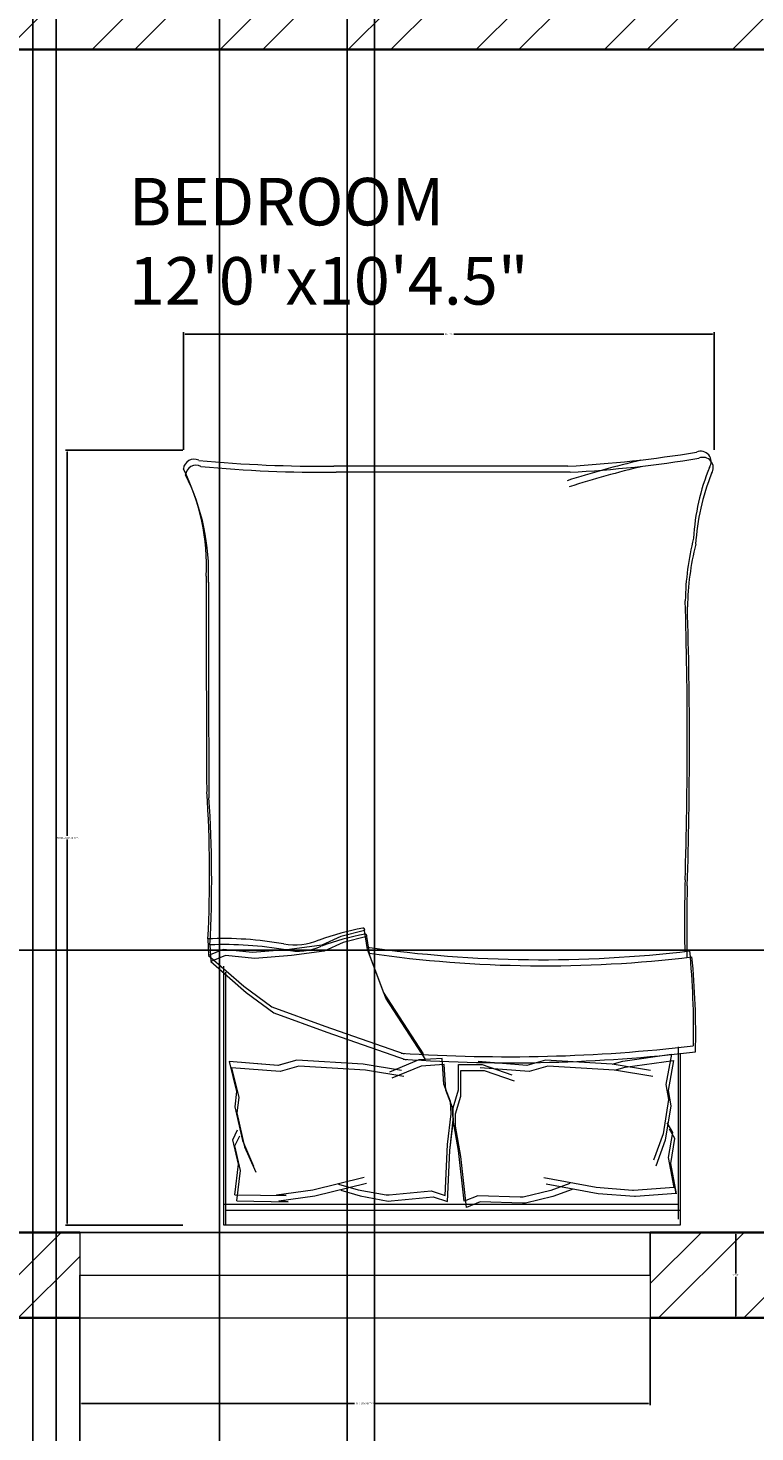
# Model space of a CAD drawing. Units: inches. Extents: x 1748 to 2382, y 1346 to 2284.
# Tile 13 of 26: x 2147 to 2223, y 1456 to 1604. Entities that reach past the tile are written whole.
import ezdxf

# ---------------------------------------------------------------- set-up
doc = ezdxf.new("R2010")
doc.units = ezdxf.units.IN
for name, color, linetype, lineweight in [('A-ANNO-DIMS', 2, 'Continuous', 18), ('A-AREA-IDEN', 7, 'Continuous', 18), ('A-FURN', 8, 'Continuous', 13), ('A-GLAZ', 191, 'Continuous', 18), ('A-WALL', 7, 'Continuous', 35), ('A-WALL-PATT', 9, 'Continuous', 13)]:
    doc.layers.add(name, color=color, linetype=linetype, lineweight=lineweight)
doc.styles.get("Standard").update_dxf_attribs({"font": 'arial.ttf'})
doc.dimstyles.get("Standard").update_dxf_attribs({"dimtxt": 0.18, "dimasz": 0.18, "dimexe": 0.18, "dimexo": 0.0625, "dimgap": 0.09, "dimtad": 0, "dimtih": 1, "dimtoh": 1, "dimdec": 4, "dimzin": 0, "dimdsep": 46, "dimtxsty": 'Standard', "dimcen": 0.09, "dimadec": 0, "dimazin": 0, "dimtfac": 1, "dimtdec": 4, "dimtofl": 0, "dimtmove": 0, "dimatfit": 3, "dimfxl": 1, "dimtolj": 1, "dimtzin": 0, "dimarcsym": 0})

# ---------------------------------------------------------------- blocks, each defined once
blk = doc.blocks.new('BED-DOUBLE')
for p, q in [((3.48, 63.33), (3.48, 81.44)), ((3.48, 63.33), (3.48, 81.44)), ((3.48, 81.44), (51.49, 81.44)), ((51.27, 81.44), (51.27, 54.83)), ((51.27, 81.44), (51.27, 54.83)), ((51.49, 81.44), (51.49, 80.8)), ((3.48, 79.91), (51.27, 79.91)), ((3.48, 79.91), (51.27, 79.91)), ((3.7, 62.69), (3.7, 80.8)), ((3.7, 62.69), (3.7, 80.8)), ((51.49, 80.8), (51.49, 54.19)), ((51.49, 80.8), (51.49, 54.19)), ((3.7, 79.27), (51.49, 79.27)), ((3.7, 79.27), (51.49, 79.27)), ((3.9, 78.11), (8.18, 78.43)), ((3.9, 78.11), (8.18, 78.43)), ((8.18, 78.43), (8.29, 78.42)), ((8.18, 78.43), (8.28, 78.42)), ((8.28, 78.42), (12.11, 78.13)), ((8.29, 78.42), (12.11, 78.13)), ((14.86, 77.69), (16.88, 78.42)), ((14.86, 77.69), (16.88, 78.42)), ((16.88, 78.42), (19.77, 79.14)), ((16.88, 78.42), (19.77, 79.14)), ((17.11, 77.78), (20, 78.5)), ((17.11, 77.78), (20, 78.5)), ((19.77, 79.14), (20.09, 79.14)), ((19.77, 79.14), (20.09, 79.14)), ((20, 78.5), (20.32, 78.5)), ((20, 78.5), (20.32, 78.5)), ((20.09, 79.14), (24.54, 78.99)), ((20.09, 79.14), (24.54, 78.99)), ((20.32, 78.5), (24.77, 78.36)), ((20.32, 78.5), (24.77, 78.36)), ((24.54, 78.99), (25.98, 79.57)), ((24.54, 78.99), (25.98, 79.57)), ((24.77, 78.36), (26.21, 78.93)), ((24.77, 78.36), (26.21, 78.93)), ((25.98, 79.57), (26.56, 74.22)), ((25.98, 79.57), (26.56, 74.22)), ((26.21, 78.93), (26.79, 73.58)), ((26.21, 78.93), (26.79, 73.58)), ((27.98, 78.95), (27.73, 73.58)), ((27.98, 78.95), (27.73, 73.58)), ((28.21, 78.31), (27.96, 72.94)), ((28.21, 78.31), (27.96, 72.94)), ((29.46, 78.46), (27.98, 78.95)), ((29.46, 78.46), (27.98, 78.95)), ((29.68, 77.83), (28.21, 78.31)), ((29.68, 77.83), (28.21, 78.31)), ((33.88, 78.89), (29.46, 78.46)), ((33.88, 78.89), (29.46, 78.46)), ((34.21, 78.91), (33.88, 78.89)), ((34.2, 78.91), (33.88, 78.89)), ((37.14, 78.37), (34.2, 78.91)), ((37.14, 78.37), (34.21, 78.91)), ((41.91, 78.37), (36.5, 77.02)), ((41.91, 78.37), (36.5, 77.02)), ((39.2, 77.77), (37.14, 78.37)), ((39.2, 77.77), (37.14, 78.37)), ((45.71, 78.9), (41.91, 78.37)), ((45.71, 78.9), (41.91, 78.37)), ((50.11, 78.89), (44.71, 78.98)), ((44.71, 78.98), (45.71, 78.9)), ((50.11, 78.89), (44.71, 78.98)), ((44.71, 78.98), (45.71, 78.9)), ((50.34, 78.25), (44.94, 78.34)), ((44.94, 78.34), (45.94, 78.26)), ((50.34, 78.25), (44.94, 78.34)), ((44.94, 78.34), (45.94, 78.26)), ((50.11, 78.89), (49.73, 75.68)), ((50.11, 78.89), (49.73, 75.68)), ((3.89, 78.13), (4.47, 74.95)), ((3.9, 78.13), (4.47, 74.95)), ((4.12, 77.49), (4.7, 74.31)), ((4.12, 77.49), (4.7, 74.31)), ((4.13, 77.47), (8.41, 77.8)), ((4.13, 77.47), (8.41, 77.8)), ((8.41, 77.8), (8.51, 77.78)), ((8.41, 77.8), (8.51, 77.78)), ((8.51, 77.78), (12.34, 77.49)), ((8.51, 77.78), (12.34, 77.49)), ((12.11, 78.13), (17.6, 77.12)), ((12.11, 78.13), (17.6, 77.12)), ((12.34, 77.49), (17.83, 76.48)), ((12.34, 77.49), (17.83, 76.48)), ((15.08, 77.05), (17.11, 77.78)), ((15.08, 77.05), (17.11, 77.78)), ((34.11, 78.25), (29.68, 77.83)), ((34.11, 78.25), (29.68, 77.83)), ((34.43, 78.27), (34.11, 78.25)), ((34.43, 78.27), (34.11, 78.25)), ((37.36, 77.73), (34.43, 78.27)), ((37.36, 77.73), (34.43, 78.27)), ((42.14, 77.73), (36.72, 76.38)), ((42.14, 77.73), (36.72, 76.38)), ((39.43, 77.13), (37.36, 77.73)), ((39.43, 77.13), (37.36, 77.73)), ((45.94, 78.26), (42.14, 77.73)), ((45.94, 78.26), (42.14, 77.73)), ((50.34, 78.25), (49.96, 75.04)), ((50.34, 78.25), (49.96, 75.04)), ((49.31, 73.19), (48.13, 75.87)), ((49.31, 73.19), (48.13, 75.87)), ((49.73, 75.68), (50.33, 73.11)), ((49.73, 75.68), (50.33, 73.11)), ((4.47, 74.95), (4.04, 72.34)), ((4.47, 74.95), (4.04, 72.34)), ((4.7, 74.31), (4.27, 71.7)), ((4.7, 74.31), (4.27, 71.7)), ((5.05, 72.49), (6.06, 75.24)), ((5.05, 72.49), (6.06, 75.24)), ((5.28, 71.85), (6.29, 74.6)), ((5.28, 71.85), (6.29, 74.6)), ((26.56, 74.22), (27.14, 71.04)), ((26.56, 74.22), (27.14, 71.04)), ((49.54, 72.55), (48.36, 75.23)), ((49.54, 72.55), (48.36, 75.23)), ((49.96, 75.04), (50.56, 72.47)), ((49.96, 75.04), (50.56, 72.47)), ((4.47, 68.87), (5.05, 72.49)), ((4.47, 68.87), (5.05, 72.49)), ((26.79, 73.58), (27.37, 70.4)), ((26.79, 73.58), (27.37, 70.4)), ((27.73, 73.58), (27.35, 70.37)), ((27.73, 73.58), (27.36, 70.37)), ((27.96, 72.94), (27.58, 69.73)), ((27.96, 72.94), (27.58, 69.73)), ((50.11, 69.61), (49.31, 73.19)), ((50.11, 69.61), (49.31, 73.19)), ((50.34, 68.98), (49.54, 72.55)), ((50.34, 68.98), (49.54, 72.55)), ((50.33, 73.11), (49.81, 72.06)), ((50.33, 73.11), (49.81, 72.06)), ((50.56, 72.47), (50.04, 71.42)), ((50.56, 72.47), (50.04, 71.42)), ((4.04, 72.34), (4.62, 71.33)), ((4.04, 72.34), (4.62, 71.33)), ((4.27, 71.7), (4.85, 70.69)), ((4.27, 71.7), (4.85, 70.69)), ((4.7, 68.23), (5.28, 71.85)), ((4.7, 68.23), (5.28, 71.85)), ((27.14, 71.04), (27.14, 69.74)), ((27.14, 71.04), (27.14, 69.74)), ((27.14, 69.74), (26.56, 67.86)), ((27.14, 69.74), (26.56, 67.86)), ((27.35, 70.37), (27.44, 69.07)), ((27.36, 70.37), (27.44, 69.07)), ((27.37, 70.4), (27.37, 69.1)), ((27.37, 70.4), (27.37, 69.1)), ((27.58, 69.73), (27.66, 68.43)), ((27.58, 69.73), (27.66, 68.43)), ((49.92, 68.01), (50.11, 69.61)), ((49.92, 68.01), (50.11, 69.61)), ((4.76, 67.28), (4.47, 68.87)), ((4.76, 67.28), (4.47, 68.87)), ((4.99, 66.64), (4.7, 68.23)), ((4.99, 66.64), (4.7, 68.23)), ((27.37, 69.1), (26.79, 67.22)), ((27.37, 69.1), (26.79, 67.22)), ((27.44, 69.07), (28.13, 67.23)), ((27.44, 69.07), (28.13, 67.23)), ((27.66, 68.43), (28.36, 66.59)), ((27.66, 68.43), (28.36, 66.59)), ((50.7, 64.87), (49.92, 68.01)), ((50.7, 64.87), (49.92, 68.01)), ((50.15, 67.37), (50.34, 68.98)), ((50.15, 67.37), (50.34, 68.98)), ((4.18, 64.1), (4.76, 67.28)), ((4.18, 64.1), (4.76, 67.28)), ((4.41, 63.46), (4.99, 66.64)), ((4.41, 63.46), (4.99, 66.64)), ((26.56, 67.86), (26.56, 65.18)), ((26.56, 67.86), (26.56, 65.18)), ((26.79, 67.22), (26.79, 64.54)), ((26.79, 67.22), (26.79, 64.54)), ((28.13, 67.23), (28.3, 64.55)), ((28.13, 67.23), (28.3, 64.55)), ((28.36, 66.59), (28.53, 63.91)), ((28.36, 66.59), (28.53, 63.91)), ((50.93, 64.23), (50.15, 67.37)), ((50.93, 64.23), (50.15, 67.37)), ((6.38, 65.81), (10.41, 65.15)), ((6.38, 65.81), (10.41, 65.15)), ((6.61, 65.18), (10.64, 64.51)), ((6.61, 65.18), (10.64, 64.51)), ((10.41, 65.15), (9.28, 64.83)), ((10.41, 65.15), (9.28, 64.83)), ((10.41, 65.15), (17.42, 64.72)), ((10.41, 65.15), (17.42, 64.72)), ((17.42, 64.72), (19.38, 65.27)), ((17.42, 64.72), (19.38, 65.27)), ((19.38, 65.27), (24.52, 64.87)), ((19.38, 65.27), (24.52, 64.87)), ((24.1, 65.18), (20.96, 66.27)), ((24.1, 65.18), (20.96, 66.27)), ((24.33, 64.54), (21.19, 65.63)), ((24.33, 64.54), (21.19, 65.63)), ((26.56, 65.18), (24.1, 65.18)), ((26.56, 65.18), (24.1, 65.18)), ((30.75, 64.7), (33.82, 65.99)), ((30.75, 64.7), (33.82, 65.99)), ((30.98, 64.06), (34.05, 65.35)), ((30.98, 64.06), (34.05, 65.35)), ((32.56, 65.81), (36.6, 65.15)), ((32.56, 65.81), (36.6, 65.15)), ((32.79, 65.18), (36.83, 64.51)), ((32.79, 65.18), (36.82, 64.51)), ((36.6, 65.15), (43.61, 64.72)), ((36.6, 65.15), (43.61, 64.72)), ((43.61, 64.72), (45.57, 65.27)), ((43.61, 64.72), (45.57, 65.27)), ((45.57, 65.27), (50.7, 64.87)), ((45.57, 65.27), (50.7, 64.87)), ((9.28, 64.83), (4.18, 64.1)), ((9.28, 64.83), (4.18, 64.1)), ((9.51, 64.19), (4.41, 63.46)), ((9.51, 64.19), (4.41, 63.46)), ((10.64, 64.51), (9.51, 64.19)), ((10.64, 64.51), (9.51, 64.19)), ((10.64, 64.51), (17.65, 64.08)), ((10.64, 64.51), (17.65, 64.08)), ((17.65, 64.08), (19.61, 64.64)), ((17.65, 64.08), (19.61, 64.64)), ((19.61, 64.64), (24.74, 64.23)), ((19.61, 64.64), (24.74, 64.23)), ((26.79, 64.54), (24.33, 64.54)), ((26.79, 64.54), (24.33, 64.54)), ((28.3, 64.55), (30.75, 64.7)), ((28.3, 64.55), (30.75, 64.7)), ((28.53, 63.91), (30.98, 64.06)), ((28.53, 63.91), (30.98, 64.06)), ((30.26, 64.06), (34.45, 57.57)), ((30.26, 64.06), (34.45, 57.57)), ((40.64, 61.13), (32.31, 64.06)), ((40.64, 61.13), (32.31, 64.06)), ((36.82, 64.51), (43.83, 64.08)), ((36.83, 64.51), (43.83, 64.08)), ((43.83, 64.08), (45.8, 64.64)), ((43.83, 64.08), (45.79, 64.64)), ((45.79, 64.64), (50.93, 64.23)), ((45.8, 64.64), (50.93, 64.23)), ((30.49, 63.42), (34.68, 56.93)), ((30.49, 63.42), (34.68, 56.93)), ((40.87, 60.49), (32.53, 63.42)), ((40.87, 60.49), (32.53, 63.42)), ((46.22, 59.11), (40.64, 61.13)), ((46.22, 59.11), (40.64, 61.13)), ((46.45, 58.48), (40.87, 60.49)), ((46.45, 58.48), (40.87, 60.49)), ((49.16, 56.95), (46.22, 59.11)), ((49.16, 56.95), (46.22, 59.11)), ((49.39, 56.31), (46.45, 58.48)), ((49.39, 56.31), (46.45, 58.48)), ((34.45, 57.57), (36.15, 53.08)), ((34.45, 57.57), (36.15, 53.08)), ((34.68, 56.93), (36.38, 52.44)), ((34.68, 56.93), (36.38, 52.44)), ((52.87, 53.7), (49.16, 56.95)), ((52.87, 53.7), (49.16, 56.95)), ((53.1, 53.06), (49.39, 56.31)), ((53.1, 53.06), (49.39, 56.31)), ((44.36, 53.08), (48.23, 53.39)), ((44.36, 53.08), (48.23, 53.39)), ((48.23, 53.39), (51.33, 53.08)), ((48.23, 53.39), (51.33, 53.08)), ((51.33, 53.08), (52.87, 53.7)), ((51.33, 53.08), (52.87, 53.7)), ((52.95, 51.95), (52.87, 53.7, 3.87)), ((52.95, 51.95), (52.87, 53.7, 3.87)), ((36.15, 53.08), (36.46, 51.07)), ((36.15, 53.08), (36.46, 51.07)), ((36.38, 52.44), (36.69, 50.43)), ((36.38, 52.44), (36.69, 50.43)), ((38.94, 51.69), (40.95, 52.61)), ((38.94, 51.69), (40.95, 52.61)), ((39.17, 51.05), (41.18, 51.97)), ((39.17, 51.05), (41.18, 51.97)), ((40.95, 52.61), (44.36, 53.08)), ((40.95, 52.61), (44.36, 53.08)), ((41.18, 51.97), (44.59, 52.44)), ((41.18, 51.97), (44.59, 52.44)), ((44.59, 52.44), (48.46, 52.75)), ((44.59, 52.44), (48.46, 52.75)), ((48.46, 52.75), (51.56, 52.44)), ((48.46, 52.75), (51.56, 52.44)), ((51.56, 52.44), (53.1, 53.06)), ((51.56, 52.44), (53.1, 53.06)), ((53.18, 51.31), (53.1, 53.06, 3.87)), ((53.18, 51.31), (53.1, 53.06, 3.87)), ((36.46, 51.07), (38.94, 51.69)), ((36.46, 51.07), (38.94, 51.69)), ((36.69, 50.43), (39.17, 51.05)), ((36.69, 50.43), (39.17, 51.05)), ((15.06, 2.2), (39.68, 2.2)), ((15.06, 2.2), (39.68, 2.2)), ((15.29, 1.56), (39.91, 1.56)), ((15.29, 1.56), (39.91, 1.56))]:
    blk.add_line(p, q)
for centre, radius, start, end in [((21.36, -100.61), 164.97, 86.0865, 96.7821), ((21.36, -100.61), 164.97, 86.0865, 96.7821), ((21.59, -101.25), 164.97, 86.0865, 96.7821), ((21.59, -101.25), 164.97, 86.0865, 96.7821), ((85.16, 61.35), 83.31, 178.7218, 185.604), ((85.16, 61.35), 83.31, 178.7218, 185.604), ((85.39, 60.71), 83.31, 178.7218, 185.604), ((85.39, 60.71), 83.31, 178.7218, 185.604), ((17.76, -74.87), 129.02, 81.7845, 96.9006), ((17.76, -74.87), 129.02, 81.7845, 96.9006), ((17.98, -75.51), 129.02, 81.7845, 96.9006), ((17.98, -75.51), 129.02, 81.7845, 96.9006), ((-167.31, 50.27), 170.11, 358.4762, 1.0082), ((-167.31, 50.27), 170.11, 358.4762, 1.0082), ((-167.08, 49.63), 170.11, 358.4762, 1.0082), ((-167.08, 49.63), 170.11, 358.4762, 1.0082), ((31.15, 79.96), 29.65, 280.6617, 289.8806), ((31.15, 79.96), 29.65, 280.6617, 289.8806), ((43.74, 46.38), 6.22, 78.6608, 113.7384), ((43.74, 46.38), 6.22, 78.6608, 113.7384), ((43.97, 45.74), 6.22, 78.6608, 113.7384), ((43.97, 45.74), 6.22, 78.6608, 113.7384), ((51.33, 88.1), 36.18, 259.8763, 272.5657), ((51.33, 88.1), 36.18, 259.8763, 272.5657), ((51.56, 87.46), 36.18, 259.8763, 272.5657), ((51.56, 87.46), 36.18, 259.8763, 272.5657), ((182.27, 45.13), 129.5, 176.9791, 183.8365), ((182.27, 45.13), 129.5, 176.9791, 183.8365), ((36.64, 51), 0.185, 160.2464, 271.1377), ((36.64, 51), 0.185, 160.2464, 271.1377), ((36.87, 50.36), 0.185, 160.2464, 271.1377), ((36.86, 50.36), 0.185, 160.2464, 271.1377), ((31.38, 79.32), 29.65, 280.6617, 289.8806), ((31.38, 79.32), 29.65, 280.6617, 289.8806), ((182.49, 44.49), 129.5, 176.9791, 183.8365), ((182.49, 44.49), 129.5, 176.9791, 183.8365), ((484.82, 30.83), 482.31, 178.2277, 181.7185), ((484.82, 30.83), 482.31, 178.2277, 181.7185), ((485.05, 30.19), 482.31, 178.2277, 181.7185), ((485.05, 30.19), 482.31, 178.2277, 181.7185), ((-4508.74, 13.62), 4561.86, 0.00217, 0.28689), ((-4508.74, 13.62), 4561.86, 0.00217, 0.28689), ((-4508.51, 12.98), 4561.86, 0.00217, 0.28689), ((-4508.51, 12.98), 4561.86, 0.00217, 0.28689), ((-26.9, 16.93), 29.63, 346.0648, 358.9113), ((-26.9, 16.93), 29.63, 346.0648, 358.9113), ((-26.67, 16.29), 29.63, 346.0648, 358.9113), ((-26.67, 16.29), 29.63, 346.0648, 358.9113), ((76.16, 12.78), 23.07, 177.4714, 206.4681), ((76.16, 12.78), 23.07, 177.4714, 206.4681), ((76.39, 12.14), 23.07, 177.4714, 206.4681), ((76.39, 12.14), 23.07, 177.4714, 206.4681), ((-21.66, 11.17), 23.56, 337.9751, 356.652), ((-21.66, 11.17), 23.56, 337.9751, 356.652), ((-21.43, 10.53), 23.56, 337.9751, 356.652), ((-21.43, 10.53), 23.56, 337.9751, 356.652), ((-17.22, 105.16), 106.46, 283.3832, 287.7053), ((-17.22, 105.16), 106.46, 283.3832, 287.7053), ((-16.99, 104.52), 106.46, 283.3832, 287.7053), ((-16.99, 104.52), 106.46, 283.3832, 287.7053), ((1.09, 1.73), 1.09, 146.1736, 293.4781), ((1.09, 1.73), 1.09, 146.1736, 293.4781), ((1.32, 1.09), 1.09, 146.1736, 293.4781), ((1.32, 1.09), 1.09, 146.1736, 293.4781), ((21.43, -119.39), 121.76, 92.9958, 99.4091), ((21.43, -119.39), 121.76, 92.9958, 99.4091), ((21.66, -120.03), 121.76, 92.9958, 99.4091), ((21.66, -120.03), 121.76, 92.9958, 99.4091), ((41.15, -130.83), 133.04, 84.4998, 90.6351), ((41.15, -130.83), 133.04, 84.4998, 90.6351), ((41.38, -131.47), 133.04, 84.4998, 90.6351), ((41.38, -131.47), 133.04, 84.4998, 90.6351), ((54.41, 2.57), 1.1, 242.6588, 356.02), ((54.41, 2.57), 1.1, 242.6588, 356.02), ((54.64, 1.93), 1.1, 242.6588, 356.02), ((54.64, 1.93), 1.1, 242.6588, 356.02)]:
    blk.add_arc(centre, radius, start, end)
blk = doc.blocks.new('WIN-60-DEEP')
for p, q in [((0, 9), (0, 0)), ((60, 9), (0, 9)), ((60, 4.5), (60, 9)), ((60, 9), (60, 0)), ((0, 0), (0, 4.5)), ((0, 4.5), (60, 4.5)), ((0, 0), (60, 0))]:
    blk.add_line(p, q)
blk = doc.blocks.new('*D12')
at = {"layer": 'A-ANNO-DIMS', "color": 0, "lineweight": -2, "transparency": 16777216}
for p, q in [((2163.18, 1559.17), (2150.83, 1559.17)), ((2151.01, 1558.99), (2151.01, 1518.58)), ((2151.01, 1477.8), (2151.01, 1518.21)), ((2163.18, 1477.62), (2150.83, 1477.62))]:
    blk.add_line(p, q, dxfattribs=at)
at = {"layer": 'A-ANNO-DIMS', "color": 0, "transparency": 16777216}
for points in [[(2150.98, 1558.99), (2151.04, 1558.99), (2151.01, 1559.17)], [(2150.98, 1477.8), (2151.04, 1477.8), (2151.01, 1477.62)]]:
    blk.add_solid(points, dxfattribs=at)
at = {"layer": 'Defpoints', "color": 0, "transparency": 16777216}
for p in [(2163.24, 1559.17), (2151.01, 1477.62), (2163.24, 1477.62)]:
    blk.add_point(p, dxfattribs=at)
at = {"layer": 'A-ANNO-DIMS', "color": 0, "transparency": 16777216, "insert": (2151.01, 1518.39), "char_height": 0.18, "attachment_point": 5}
blk.add_mtext('\\A1;DOUBLE BED 82 TYP.', dxfattribs=at)
blk = doc.blocks.new('*D13')
at = {"layer": 'A-ANNO-DIMS', "color": 0, "lineweight": -2, "transparency": 16777216}
for p, q in [((2163.24, 1559.23), (2163.24, 1571.58)), ((2163.42, 1571.4), (2190.63, 1571.4)), ((2218.89, 1571.4), (2191.68, 1571.4)), ((2219.07, 1559.23), (2219.07, 1571.58))]:
    blk.add_line(p, q, dxfattribs=at)
at = {"layer": 'A-ANNO-DIMS', "color": 0, "transparency": 16777216}
for points in [[(2163.42, 1571.43), (2163.42, 1571.37), (2163.24, 1571.4)], [(2218.89, 1571.43), (2218.89, 1571.37), (2219.07, 1571.4)]]:
    blk.add_solid(points, dxfattribs=at)
at = {"layer": 'Defpoints', "color": 0, "transparency": 16777216}
for p in [(2163.24, 1571.4), (2163.24, 1559.17), (2219.07, 1559.17)]:
    blk.add_point(p, dxfattribs=at)
at = {"layer": 'A-ANNO-DIMS', "color": 0, "transparency": 16777216, "insert": (2191.16, 1571.4), "char_height": 0.18, "attachment_point": 5}
blk.add_mtext('\\A1;56 TYP.', dxfattribs=at)
blk = doc.blocks.new('*D26')
at = {"layer": 'A-ANNO-DIMS', "color": 0, "lineweight": -2, "transparency": 16777216}
for p, q in [((2152.34, 1467.79), (2152.34, 1458.67)), ((2212.34, 1467.79), (2212.34, 1458.67)), ((2152.52, 1458.85), (2181.22, 1458.85)), ((2212.16, 1458.85), (2183.45, 1458.85))]:
    blk.add_line(p, q, dxfattribs=at)
at = {"layer": 'A-ANNO-DIMS', "color": 0, "transparency": 16777216}
for points in [[(2152.52, 1458.88), (2152.52, 1458.82), (2152.34, 1458.85)], [(2212.16, 1458.88), (2212.16, 1458.82), (2212.34, 1458.85)]]:
    blk.add_solid(points, dxfattribs=at)
at = {"layer": 'Defpoints', "color": 0, "transparency": 16777216}
for p in [(2152.34, 1467.85), (2212.34, 1467.85), (2212.34, 1458.85)]:
    blk.add_point(p, dxfattribs=at)
at = {"layer": 'A-ANNO-DIMS', "color": 0, "transparency": 16777216, "insert": (2182.34, 1458.85), "char_height": 0.18, "attachment_point": 5}
blk.add_mtext('\\A1;WINDOW 60 TYP.', dxfattribs=at)
blk = doc.blocks.new('*D27')
at = {"layer": 'A-ANNO-DIMS', "color": 0, "lineweight": -2, "transparency": 16777216}
for p, q in [((2212.4, 1476.85), (2221.52, 1476.85)), ((2221.34, 1476.67), (2221.34, 1472.53)), ((2221.34, 1468.03), (2221.34, 1472.17)), ((2212.4, 1467.85), (2221.52, 1467.85))]:
    blk.add_line(p, q, dxfattribs=at)
at = {"layer": 'A-ANNO-DIMS', "color": 0, "transparency": 16777216}
for points in [[(2221.31, 1476.67), (2221.37, 1476.67), (2221.34, 1476.85)], [(2221.31, 1468.03), (2221.37, 1468.03), (2221.34, 1467.85)]]:
    blk.add_solid(points, dxfattribs=at)
at = {"layer": 'Defpoints', "color": 0, "transparency": 16777216}
for p in [(2212.34, 1476.85), (2221.34, 1476.85), (2212.34, 1467.85)]:
    blk.add_point(p, dxfattribs=at)
at = {"layer": 'A-ANNO-DIMS', "color": 0, "transparency": 16777216, "insert": (2221.34, 1472.35), "char_height": 0.18, "attachment_point": 5}
blk.add_mtext('\\A1;9 TYP.', dxfattribs=at)
blk = doc.blocks.new('*D46')
at = {"layer": 'A-ANNO-DIMS', "color": 0, "lineweight": -2, "transparency": 16777216}
for p, q in [((2147.39, 1725.79), (2147.39, 1360.47)), ((2180.46, 1725.79), (2180.46, 1360.47)), ((2147.57, 1360.65), (2163.46, 1360.65)), ((2180.28, 1360.65), (2164.39, 1360.65))]:
    blk.add_line(p, q, dxfattribs=at)
at = {"layer": 'A-ANNO-DIMS', "color": 0, "transparency": 16777216}
for points in [[(2147.57, 1360.68), (2147.57, 1360.62), (2147.39, 1360.65)], [(2180.28, 1360.68), (2180.28, 1360.62), (2180.46, 1360.65)]]:
    blk.add_solid(points, dxfattribs=at)
at = {"layer": 'Defpoints', "color": 0, "transparency": 16777216}
for p in [(2147.39, 1725.85), (2180.46, 1725.85), (2180.46, 1360.65)]:
    blk.add_point(p, dxfattribs=at)
at = {"layer": 'A-ANNO-DIMS', "color": 0, "transparency": 16777216, "insert": (2163.92, 1360.65), "char_height": 0.18, "attachment_point": 5}
blk.add_mtext('\\A1;33.066', dxfattribs=at)
blk = doc.blocks.new('*D47')
at = {"layer": 'A-ANNO-DIMS', "color": 0, "lineweight": -2, "transparency": 16777216}
for p, q in [((2149.85, 1913.29), (2149.85, 1360.47)), ((2183.35, 1913.29), (2183.35, 1360.47)), ((2150.03, 1360.65), (2166.28, 1360.65)), ((2183.17, 1360.65), (2166.93, 1360.65))]:
    blk.add_line(p, q, dxfattribs=at)
at = {"layer": 'A-ANNO-DIMS', "color": 0, "transparency": 16777216}
for points in [[(2150.03, 1360.68), (2150.03, 1360.62), (2149.85, 1360.65)], [(2183.17, 1360.68), (2183.17, 1360.62), (2183.35, 1360.65)]]:
    blk.add_solid(points, dxfattribs=at)
at = {"layer": 'Defpoints', "color": 0, "transparency": 16777216}
for p in [(2149.85, 1913.35), (2183.35, 1913.35), (2183.35, 1360.65)]:
    blk.add_point(p, dxfattribs=at)
at = {"layer": 'A-ANNO-DIMS', "color": 0, "transparency": 16777216, "insert": (2166.6, 1360.65), "char_height": 0.18, "attachment_point": 5}
blk.add_mtext('\\A1;33.5', dxfattribs=at)
blk = doc.blocks.new('*D53')
at = {"layer": 'A-ANNO-DIMS', "color": 0, "lineweight": -2, "transparency": 16777216}
for p, q in [((2115.4, 2223.79), (2115.4, 1360.47)), ((2167.02, 2223.79), (2167.02, 1360.47)), ((2115.58, 1360.65), (2140.81, 1360.65)), ((2166.84, 1360.65), (2141.6, 1360.65))]:
    blk.add_line(p, q, dxfattribs=at)
at = {"layer": 'A-ANNO-DIMS', "color": 0, "transparency": 16777216}
for points in [[(2115.58, 1360.68), (2115.58, 1360.62), (2115.4, 1360.65)], [(2166.84, 1360.68), (2166.84, 1360.62), (2167.02, 1360.65)]]:
    blk.add_solid(points, dxfattribs=at)
at = {"layer": 'Defpoints', "color": 0, "transparency": 16777216}
for p in [(2115.4, 2223.85), (2167.02, 2223.85), (2167.02, 1360.65)]:
    blk.add_point(p, dxfattribs=at)
at = {"layer": 'A-ANNO-DIMS', "color": 0, "transparency": 16777216, "insert": (2141.21, 1360.65), "char_height": 0.18, "attachment_point": 5}
blk.add_mtext('\\A1;51.62', dxfattribs=at)
blk = doc.blocks.new('*D54')
at = {"layer": 'A-ANNO-DIMS', "color": 0, "lineweight": -2, "transparency": 16777216}
for p, q in [((2288.4, 1506.57), (1779.88, 1506.57)), ((1780.06, 1506.39), (1780.06, 1491.89)), ((1780.06, 1477.03), (1780.06, 1491.53)), ((2288.4, 1476.85), (1779.88, 1476.85))]:
    blk.add_line(p, q, dxfattribs=at)
at = {"layer": 'A-ANNO-DIMS', "color": 0, "transparency": 16777216}
for points in [[(1780.03, 1506.39), (1780.09, 1506.39), (1780.06, 1506.57)], [(1780.03, 1477.03), (1780.09, 1477.03), (1780.06, 1476.85)]]:
    blk.add_solid(points, dxfattribs=at)
at = {"layer": 'Defpoints', "color": 0, "transparency": 16777216}
for p in [(1780.06, 1506.57), (2288.46, 1506.57), (2288.46, 1476.85)]:
    blk.add_point(p, dxfattribs=at)
at = {"layer": 'A-ANNO-DIMS', "color": 0, "transparency": 16777216, "insert": (1780.06, 1491.71), "char_height": 0.18, "attachment_point": 5}
blk.add_mtext('\\A1;29.716', dxfattribs=at)
blk = doc.blocks.new('*D67')
at = {"layer": 'A-ANNO-DIMS', "color": 0, "lineweight": -2, "transparency": 16777216}
for p, q in [((2095.36, 1467.79), (2095.36, 1360.47)), ((2152.34, 1467.79), (2152.34, 1360.47)), ((2095.54, 1360.65), (2123.45, 1360.65)), ((2152.16, 1360.65), (2124.24, 1360.65))]:
    blk.add_line(p, q, dxfattribs=at)
at = {"layer": 'A-ANNO-DIMS', "color": 0, "transparency": 16777216}
for points in [[(2095.54, 1360.68), (2095.54, 1360.62), (2095.36, 1360.65)], [(2152.16, 1360.68), (2152.16, 1360.62), (2152.34, 1360.65)]]:
    blk.add_solid(points, dxfattribs=at)
at = {"layer": 'Defpoints', "color": 0, "transparency": 16777216}
for p in [(2095.36, 1467.85), (2152.34, 1467.85), (2152.34, 1360.65)]:
    blk.add_point(p, dxfattribs=at)
at = {"layer": 'A-ANNO-DIMS', "color": 0, "transparency": 16777216, "insert": (2123.85, 1360.65), "char_height": 0.18, "attachment_point": 5}
blk.add_mtext('\\A1;56.97', dxfattribs=at)

msp = doc.modelspace()

# ---------------------------------------------------------------- hatches: boundary and pattern name
at = {"layer": 'A-WALL-PATT'}
h = msp.add_hatch(dxfattribs=at)
h.set_pattern_fill('ANSI32', color=256)
h.paths.add_polyline_path([(1908.4445, 2232.8497), (1821.9607, 2232.8497), (1821.9607, 2223.8497), (1865.4607, 2223.8497), (1865.4607, 2209.9185), (1869.9607, 2209.9185), (1869.9607, 2223.8497), (1908.4445, 2223.8497), (1908.4445, 2228.3497)])
h.paths.add_polyline_path([(2040.0683, 2232.8497), (1968.4445, 2232.8497), (1968.4445, 2223.8497), (2025.9607, 2223.8497), (2025.9607, 2130.3497), (2032.1341, 2130.3497), (2032.1341, 2132.5997), (2032.1341, 2134.8497), (2030.4607, 2134.8497), (2030.4607, 2223.8497), (2040.0683, 2223.8497)])
h.paths.add_polyline_path([(2091.3969, 2232.8497), (2064.0683, 2232.8497), (2064.0683, 2223.8497), (2078.4607, 2223.8497), (2078.4607, 2134.8497), (2051.1563, 2134.8497), (2051.1563, 2130.3497), (2078.4607, 2130.3497), (2078.4607, 2128.6813), (2082.9607, 2128.6813), (2082.9607, 2130.3497), (2086.1879, 2130.3497), (2086.1879, 2132.5997), (2086.1879, 2134.8497), (2082.9607, 2134.8497), (2082.9607, 2223.8497), (2091.3969, 2223.8497), (2091.3969, 2228.3497)])
h.paths.add_polyline_path([(2167.0164, 2232.8497), (2115.3969, 2232.8497), (2115.3969, 2223.8497), (2130.9607, 2223.8497), (2130.9607, 2134.8497), (2106.9607, 2134.8497), (2106.9607, 2130.3497), (2135.4607, 2130.3497), (2135.4607, 2223.8497), (2167.0164, 2223.8497), (2167.0164, 2228.3497)])
h.paths.add_polyline_path([(1869.9607, 2149.9185), (1865.4607, 2149.9185), (1865.4607, 2127.8942), (1869.9607, 2127.8942)])
h.paths.add_polyline_path([(2082.9607, 2104.4871), (2080.7107, 2104.4871), (2078.4607, 2104.4871), (2078.4607, 2103.8497), (1869.9607, 2103.8497), (1869.9607, 2108.6062), (1867.7107, 2108.6062), (1865.4607, 2108.6062), (1865.4607, 2103.8497), (1821.9607, 2103.8497), (1821.9607, 2099.3497), (1865.4607, 2099.3497), (1865.4607, 2094.7509), (1869.9607, 2094.7509), (1869.9607, 2099.3497), (2025.9607, 2099.3497), (2025.9607, 2096.4326), (2030.4607, 2096.4326), (2030.4607, 2099.3497), (2082.9607, 2099.3497)])
h.paths.add_polyline_path([(1928.9457, 1401.1212), (2176.8693, 1401.1212), (2176.8693, 1438.214), (1928.9457, 1438.214)], flags=9)
h.paths.add_polyline_path([(2122.2668, 2048.1927), (2177.9387, 2048.1927), (2177.9387, 2066.85), (2122.2668, 2066.85)], flags=9)
h.paths.add_polyline_path([(2272.688, 2153.8197), (2272.688, 2216.746), (2262.3845, 2216.746), (2262.3845, 2153.8197)], flags=9)
h.paths.add_polyline_path([(2157.2928, 2166.5593), (2196.3822, 2166.5593), (2196.3822, 2185.2167), (2157.2928, 2185.2167)], flags=9)
h.paths.add_polyline_path([(2089.3407, 2162.0698), (2124.3987, 2162.0698), (2124.3987, 2180.7272), (2089.3407, 2180.7272)], flags=9)
h.paths.add_polyline_path([(2037.4521, 2160.0913), (2072.5101, 2160.0913), (2072.5101, 2178.7486), (2037.4521, 2178.7486)], flags=9)
h.paths.add_polyline_path([(1884.7894, 2104.1554), (1923.6297, 2104.1554), (1923.6297, 2122.8127), (1884.7894, 2122.8127)], flags=9)
h.paths.add_polyline_path([(1851.2832, 2142.9749), (1851.2832, 2199.3051), (1840.9796, 2199.3051), (1840.9796, 2142.9749)], flags=9)
h.paths.add_polyline_path([(1844.8763, 2017.2834), (1844.8763, 2073.6136), (1834.5728, 2073.6136), (1834.5728, 2017.2834)], flags=9)
h.paths.add_polyline_path([(1897.1577, 2073.1279), (1935.9981, 2073.1279), (1935.9981, 2091.7853), (1897.1577, 2091.7853)], flags=9)
h.paths.add_polyline_path([(1952.3395, 1802.4231), (2008.0114, 1802.4231), (2008.0114, 1821.0805), (1952.3395, 1821.0805)], flags=9)
h.paths.add_polyline_path([(1978.8184, 1857.6841), (2017.7338, 1857.6841), (2017.7338, 1876.3415), (1978.8184, 1876.3415)], flags=9)
h.paths.add_polyline_path([(1979.6513, 1925.9516), (2008.8089, 1925.9516), (2008.8089, 1944.6089), (1979.6513, 1944.6089)], flags=9)
h.paths.add_polyline_path([(1838.5553, 1860.3527), (1877.3957, 1860.3527), (1877.3957, 1879.01), (1838.5553, 1879.01)], flags=9)
h.paths.add_polyline_path([(1883.9018, 1787.3013), (1883.9018, 1843.6315), (1873.5983, 1843.6315), (1873.5983, 1787.3013)], flags=9)
h.paths.add_polyline_path([(1873.7079, 1509.1938), (1873.7079, 1583.7709), (1863.4044, 1583.7709), (1863.4044, 1509.1938)], flags=9)
h.paths.add_polyline_path([(1916.2259, 1603.3681), (1955.0663, 1603.3681), (1955.0663, 1622.0254), (1916.2259, 1622.0254)], flags=9)
h.paths.add_polyline_path([(1876.3013, 1636.757), (1876.3013, 1693.0871), (1865.9978, 1693.0871), (1865.9978, 1636.757)], flags=9)
h.paths.add_polyline_path([(1921.3138, 1521.8316), (1964.0662, 1521.8316), (1964.0662, 1540.489), (1921.3138, 1540.489)], flags=9)
h.paths.add_polyline_path([(2017.5657, 1497.5078), (2046.7983, 1497.5078), (2046.7983, 1516.1651), (2017.5657, 1516.1651)], flags=9)
h.paths.add_polyline_path([(2066.8661, 1499.3902), (2096.0988, 1499.3902), (2096.0988, 1518.0475), (2066.8661, 1518.0475)], flags=9)
h.paths.add_polyline_path([(2155.4835, 1571.6596), (2198.2358, 1571.6596), (2198.2358, 1590.3169), (2155.4835, 1590.3169)], flags=9)
h.paths.add_polyline_path([(2094.9136, 1664.6812), (2150.5855, 1664.6812), (2150.5855, 1683.3386), (2094.9136, 1683.3386)], flags=9)
h.paths.add_polyline_path([(2257.6902, 1863.1628), (2269.8935, 1863.1628), (2269.8935, 1873.4664), (2257.6902, 1873.4664)], flags=9)
h.paths.add_polyline_path([(2164.0748, 1880.3089), (2189.8694, 1880.3089), (2189.8694, 1890.6124), (2164.0748, 1890.6124)], flags=9)
h.paths.add_polyline_path([(2239.4394, 1931.0585), (2268.8187, 1931.0585), (2268.8187, 1949.7159), (2239.4394, 1949.7159)], flags=9)
h = msp.add_hatch(dxfattribs=at)
h.set_pattern_fill('ANSI32', color=256)
h.paths.add_polyline_path([(2297.4607, 2232.8497), (2203.0164, 2232.8497), (2203.0164, 2223.8497), (2244.9607, 2223.8497), (2244.9607, 2127.8554), (2249.4607, 2127.8554), (2249.4607, 2223.8497), (2297.4607, 2223.8497)])
h.paths.add_polyline_path([(2297.4607, 2103.8497), (2249.4607, 2103.8497), (2249.4607, 2106.7497), (2247.2107, 2106.7497), (2244.9607, 2106.7497), (2244.9607, 2103.8497), (2130.9607, 2103.8497), (2130.9607, 2099.3497), (2288.4607, 2099.3497), (2288.4607, 2077.2008), (2297.4607, 2077.2008)])
h.paths.add_polyline_path([(1928.9457, 1401.1212), (2176.8693, 1401.1212), (2176.8693, 1438.214), (1928.9457, 1438.214)], flags=9)
h.paths.add_polyline_path([(2122.2668, 2048.1927), (2177.9387, 2048.1927), (2177.9387, 2066.85), (2122.2668, 2066.85)], flags=9)
h.paths.add_polyline_path([(2272.688, 2153.8197), (2272.688, 2216.746), (2262.3845, 2216.746), (2262.3845, 2153.8197)], flags=25)
h.paths.add_polyline_path([(2157.2928, 2166.5593), (2196.3822, 2166.5593), (2196.3822, 2185.2167), (2157.2928, 2185.2167)], flags=9)
h.paths.add_polyline_path([(2089.3407, 2162.0698), (2124.3987, 2162.0698), (2124.3987, 2180.7272), (2089.3407, 2180.7272)], flags=9)
h.paths.add_polyline_path([(2037.4521, 2160.0913), (2072.5101, 2160.0913), (2072.5101, 2178.7486), (2037.4521, 2178.7486)], flags=9)
h.paths.add_polyline_path([(1884.7894, 2104.1554), (1923.6297, 2104.1554), (1923.6297, 2122.8127), (1884.7894, 2122.8127)], flags=9)
h.paths.add_polyline_path([(1851.2832, 2142.9749), (1851.2832, 2199.3051), (1840.9796, 2199.3051), (1840.9796, 2142.9749)], flags=9)
h.paths.add_polyline_path([(1844.8763, 2017.2834), (1844.8763, 2073.6136), (1834.5728, 2073.6136), (1834.5728, 2017.2834)], flags=9)
h.paths.add_polyline_path([(1897.1577, 2073.1279), (1935.9981, 2073.1279), (1935.9981, 2091.7853), (1897.1577, 2091.7853)], flags=9)
h.paths.add_polyline_path([(1952.3395, 1802.4231), (2008.0114, 1802.4231), (2008.0114, 1821.0805), (1952.3395, 1821.0805)], flags=9)
h.paths.add_polyline_path([(1978.8184, 1857.6841), (2017.7338, 1857.6841), (2017.7338, 1876.3415), (1978.8184, 1876.3415)], flags=9)
h.paths.add_polyline_path([(1979.6513, 1925.9516), (2008.8089, 1925.9516), (2008.8089, 1944.6089), (1979.6513, 1944.6089)], flags=9)
h.paths.add_polyline_path([(1838.5553, 1860.3527), (1877.3957, 1860.3527), (1877.3957, 1879.01), (1838.5553, 1879.01)], flags=9)
h.paths.add_polyline_path([(1883.9018, 1787.3013), (1883.9018, 1843.6315), (1873.5983, 1843.6315), (1873.5983, 1787.3013)], flags=9)
h.paths.add_polyline_path([(1873.7079, 1509.1938), (1873.7079, 1583.7709), (1863.4044, 1583.7709), (1863.4044, 1509.1938)], flags=9)
h.paths.add_polyline_path([(1916.2259, 1603.3681), (1955.0663, 1603.3681), (1955.0663, 1622.0254), (1916.2259, 1622.0254)], flags=9)
h.paths.add_polyline_path([(1876.3013, 1636.757), (1876.3013, 1693.0871), (1865.9978, 1693.0871), (1865.9978, 1636.757)], flags=9)
h.paths.add_polyline_path([(1921.3138, 1521.8316), (1964.0662, 1521.8316), (1964.0662, 1540.489), (1921.3138, 1540.489)], flags=9)
h.paths.add_polyline_path([(2017.5657, 1497.5078), (2046.7983, 1497.5078), (2046.7983, 1516.1651), (2017.5657, 1516.1651)], flags=9)
h.paths.add_polyline_path([(2066.8661, 1499.3902), (2096.0988, 1499.3902), (2096.0988, 1518.0475), (2066.8661, 1518.0475)], flags=9)
h.paths.add_polyline_path([(2155.4835, 1571.6596), (2198.2358, 1571.6596), (2198.2358, 1590.3169), (2155.4835, 1590.3169)], flags=9)
h.paths.add_polyline_path([(2094.9136, 1664.6812), (2150.5855, 1664.6812), (2150.5855, 1683.3386), (2094.9136, 1683.3386)], flags=9)
h.paths.add_polyline_path([(2257.6902, 1863.1628), (2269.8935, 1863.1628), (2269.8935, 1873.4664), (2257.6902, 1873.4664)], flags=9)
h.paths.add_polyline_path([(2164.0748, 1880.3089), (2189.8694, 1880.3089), (2189.8694, 1890.6124), (2164.0748, 1890.6124)], flags=9)
h.paths.add_polyline_path([(2239.4394, 1931.0585), (2268.8187, 1931.0585), (2268.8187, 1949.7159), (2239.4394, 1949.7159)], flags=9)
h = msp.add_hatch(dxfattribs=at)
h.set_pattern_fill('ANSI32', color=256)
h.paths.add_polyline_path([(1919.6777, 1476.8497), (1900.6426, 1476.8497), (1900.6426, 1522.0826), (1898.3926, 1522.0826), (1896.1426, 1522.0826), (1896.1426, 1476.8497), (1857.1426, 1476.8497), (1857.1426, 1467.8497), (1896.1426, 1467.8497), (1919.6777, 1467.8497), (1919.6777, 1472.3497)])
h.paths.add_polyline_path([(2018.7873, 1472.3497), (2018.7873, 1476.8497), (2010.9607, 1476.8497), (2010.9607, 1560.8497), (2034.9607, 1560.8497), (2034.9607, 1565.3497), (2006.4607, 1565.3497), (2006.4607, 1476.8497), (1955.6777, 1476.8497), (1955.6777, 1467.8497), (2018.7873, 1467.8497)])
h.paths.add_polyline_path([(2152.3354, 1472.3497), (2152.3354, 1476.8497), (2115.9607, 1476.8497), (2115.9607, 1565.3497), (2109.2204, 1565.3497), (2109.2204, 1563.0997), (2109.2204, 1560.8497), (2111.4607, 1560.8497), (2111.4607, 1476.8497), (2095.3617, 1476.8497), (2095.3617, 1467.8497), (2152.3354, 1467.8497)])
h.paths.add_polyline_path([(2071.3617, 1476.8497), (2063.4607, 1476.8497), (2063.4607, 1560.8497), (2090.1865, 1560.8497), (2090.1865, 1565.3497), (2063.4607, 1565.3497), (2063.4607, 1572.5485), (2061.2107, 1572.5485), (2058.9607, 1572.5485), (2058.9607, 1565.3497), (2055.6281, 1565.3497), (2055.6281, 1560.8497), (2058.9607, 1560.8497), (2058.9607, 1476.8497), (2042.7873, 1476.8497), (2042.7873, 1467.8497), (2071.3617, 1467.8497), (2071.3617, 1472.3497)])
h.paths.add_polyline_path([(2297.4607, 1506.5652), (2288.4607, 1506.5652), (2288.4607, 1476.8497), (2212.3354, 1476.8497), (2212.3354, 1467.8497), (2297.4607, 1467.8497)])
h.paths.add_polyline_path([(2297.4607, 1645.3038), (2288.4607, 1645.3038), (2288.4607, 1605.8497), (2058.9607, 1605.8497), (2058.9607, 1600.1857), (2061.2107, 1600.1857), (2063.4607, 1600.1857), (2063.4607, 1601.3497), (2288.4607, 1601.3497), (2288.4607, 1566.5652), (2297.4607, 1566.5652)])
h.paths.add_polyline_path([(2010.9607, 1609.0561), (2008.7107, 1609.0561), (2006.4607, 1609.0561), (2006.4607, 1605.8497), (1900.6426, 1605.8497), (1900.6426, 1609.7171), (1898.3926, 1609.7171), (1896.1426, 1609.7171), (1896.1426, 1605.8497), (1857.1426, 1605.8497), (1857.1426, 1601.3497), (1896.1426, 1601.3497), (1896.1426, 1542.5447), (1900.6426, 1542.5447), (1900.6426, 1601.3497), (2010.9607, 1601.3497)])
h.paths.add_polyline_path([(1928.9457, 1401.1212), (2176.8693, 1401.1212), (2176.8693, 1438.214), (1928.9457, 1438.214)], flags=9)
h.paths.add_polyline_path([(2122.2668, 2048.1927), (2177.9387, 2048.1927), (2177.9387, 2066.85), (2122.2668, 2066.85)], flags=9)
h.paths.add_polyline_path([(2272.688, 2153.8197), (2272.688, 2216.746), (2262.3845, 2216.746), (2262.3845, 2153.8197)], flags=9)
h.paths.add_polyline_path([(2157.2928, 2166.5593), (2196.3822, 2166.5593), (2196.3822, 2185.2167), (2157.2928, 2185.2167)], flags=9)
h.paths.add_polyline_path([(2089.3407, 2162.0698), (2124.3987, 2162.0698), (2124.3987, 2180.7272), (2089.3407, 2180.7272)], flags=9)
h.paths.add_polyline_path([(2037.4521, 2160.0913), (2072.5101, 2160.0913), (2072.5101, 2178.7486), (2037.4521, 2178.7486)], flags=9)
h.paths.add_polyline_path([(1884.7894, 2104.1554), (1923.6297, 2104.1554), (1923.6297, 2122.8127), (1884.7894, 2122.8127)], flags=9)
h.paths.add_polyline_path([(1851.2832, 2142.9749), (1851.2832, 2199.3051), (1840.9796, 2199.3051), (1840.9796, 2142.9749)], flags=9)
h.paths.add_polyline_path([(1844.8763, 2017.2834), (1844.8763, 2073.6136), (1834.5728, 2073.6136), (1834.5728, 2017.2834)], flags=9)
h.paths.add_polyline_path([(1897.1577, 2073.1279), (1935.9981, 2073.1279), (1935.9981, 2091.7853), (1897.1577, 2091.7853)], flags=9)
h.paths.add_polyline_path([(1952.3395, 1802.4231), (2008.0114, 1802.4231), (2008.0114, 1821.0805), (1952.3395, 1821.0805)], flags=9)
h.paths.add_polyline_path([(1978.8184, 1857.6841), (2017.7338, 1857.6841), (2017.7338, 1876.3415), (1978.8184, 1876.3415)], flags=9)
h.paths.add_polyline_path([(1979.6513, 1925.9516), (2008.8089, 1925.9516), (2008.8089, 1944.6089), (1979.6513, 1944.6089)], flags=9)
h.paths.add_polyline_path([(1838.5553, 1860.3527), (1877.3957, 1860.3527), (1877.3957, 1879.01), (1838.5553, 1879.01)], flags=9)
h.paths.add_polyline_path([(1883.9018, 1787.3013), (1883.9018, 1843.6315), (1873.5983, 1843.6315), (1873.5983, 1787.3013)], flags=9)
h.paths.add_polyline_path([(1873.7079, 1509.1938), (1873.7079, 1583.7709), (1863.4044, 1583.7709), (1863.4044, 1509.1938)], flags=9)
h.paths.add_polyline_path([(1916.2259, 1603.3681), (1955.0663, 1603.3681), (1955.0663, 1622.0254), (1916.2259, 1622.0254)], flags=9)
h.paths.add_polyline_path([(1876.3013, 1636.757), (1876.3013, 1693.0871), (1865.9978, 1693.0871), (1865.9978, 1636.757)], flags=9)
h.paths.add_polyline_path([(1921.3138, 1521.8316), (1964.0662, 1521.8316), (1964.0662, 1540.489), (1921.3138, 1540.489)], flags=9)
h.paths.add_polyline_path([(2017.5657, 1497.5078), (2046.7983, 1497.5078), (2046.7983, 1516.1651), (2017.5657, 1516.1651)], flags=9)
h.paths.add_polyline_path([(2066.8661, 1499.3902), (2096.0988, 1499.3902), (2096.0988, 1518.0475), (2066.8661, 1518.0475)], flags=9)
h.paths.add_polyline_path([(2155.4835, 1571.6596), (2198.2358, 1571.6596), (2198.2358, 1590.3169), (2155.4835, 1590.3169)], flags=25)
h.paths.add_polyline_path([(2094.9136, 1664.6812), (2150.5855, 1664.6812), (2150.5855, 1683.3386), (2094.9136, 1683.3386)], flags=9)
h.paths.add_polyline_path([(2257.6902, 1863.1628), (2269.8935, 1863.1628), (2269.8935, 1873.4664), (2257.6902, 1873.4664)], flags=9)
h.paths.add_polyline_path([(2164.0748, 1880.3089), (2189.8694, 1880.3089), (2189.8694, 1890.6124), (2164.0748, 1890.6124)], flags=9)
h.paths.add_polyline_path([(2239.4394, 1931.0585), (2268.8187, 1931.0585), (2268.8187, 1949.7159), (2239.4394, 1949.7159)], flags=9)

# ---------------------------------------------------------------- linework, layer by layer
at = {"layer": 'A-WALL'}
for p, q in [((2063.4607, 1601.3497), (2288.4607, 1601.3497)), ((2115.9607, 1476.8497), (2152.3354, 1476.8497)), ((2212.3354, 1476.8497), (2288.4607, 1476.8497)), ((2095.3617, 1467.8497), (2152.3354, 1467.8497)), ((2212.3354, 1467.8497), (2297.4607, 1467.8497))]:
    msp.add_line(p, q, dxfattribs=at)

# ---------------------------------------------------------------- block references
at = {"layer": 'A-FURN', "rotation": 180}
msp.add_blockref('BED-DOUBLE', (2218.9825, 1559.0637), dxfattribs=at)
at = {"layer": 'A-GLAZ'}
msp.add_blockref('WIN-60-DEEP', (2152.335, 1467.85), dxfattribs=at)

# ---------------------------------------------------------------- texts
at = {"layer": 'A-AREA-IDEN', "insert": (2157.494, 1587.8322), "char_height": 5, "attachment_point": 1}
msp.add_mtext_dynamic_manual_height_columns('BEDROOM\\P12\'0"x10\'4.5"', width=231.739709, gutter_width=12.5, heights=[0], dxfattribs=at)

# ---------------------------------------------------------------- dimensions: what is measured, and where the dimension line sits
at = {"layer": 'A-ANNO-DIMS'}
for base, p1, p2, override, picture, middle in [((2167.0164, 1360.6451), (2115.3969, 2223.8497), (2167.0164, 2223.8497), {"dimdec": 2, "dimlfac": 1, "dimrnd": 0, "dimzin": 0, "dimdsep": 46, "dimlunit": 2}, '*D53', (2141.2066, 1360.6451)), ((2183.3516, 1360.6451), (2149.8497, 1913.3497), (2183.3516, 1913.3497), {"dimdec": 1, "dimlfac": 1, "dimrnd": 0, "dimzin": 0, "dimdsep": 46, "dimlunit": 2}, '*D47', (2166.6006, 1360.6451)), ((2180.4551, 1360.6451), (2147.389, 1725.8497), (2180.4551, 1725.8497), {"dimdec": 3, "dimlfac": 1, "dimrnd": 0, "dimzin": 0, "dimdsep": 46, "dimlunit": 2}, '*D46', (2163.9221, 1360.6451)), ((2152.3354, 1360.6451), (2095.3617, 1467.8497), (2152.3354, 1467.8497), {"dimdec": 2, "dimlfac": 1, "dimrnd": 0, "dimzin": 0, "dimdsep": 46, "dimlunit": 2}, '*D67', (2123.8486, 1360.6451))]:
    dim = msp.add_linear_dim(base=base, p1=p1, p2=p2, dimstyle='Standard', override=override, dxfattribs=at)
    dim.commit()
    dim.dimension.update_dxf_attribs({"geometry": picture, "text_midpoint": middle})
for base, p1, p2, angle, text, picture, middle in [((2163.244, 1571.4011), (2219.0686, 1559.1688), (2163.244, 1559.1688), 180, '<> TYP.', '*D13', (2191.1563, 1571.4011)), ((2151.0117, 1477.6202), (2163.244, 1559.1688), (2163.244, 1477.6202), 270, 'DOUBLE BED <> TYP.', '*D12', (2151.0117, 1518.3945)), ((2221.3354, 1476.8497), (2212.3354, 1467.8497), (2212.3354, 1476.8497), 90, '<> TYP.', '*D27', (2221.3354, 1472.3497))]:
    dim = msp.add_linear_dim(base=base, p1=p1, p2=p2, angle=angle, text=text, dimstyle='Standard', override={"dimdec": 0, "dimlfac": 1, "dimrnd": 0, "dimzin": 0, "dimdsep": 46, "dimlunit": 2}, dxfattribs=at)
    dim.commit()
    dim.dimension.update_dxf_attribs({"geometry": picture, "text_midpoint": middle})
dim = msp.add_linear_dim(base=(1780.06066, 1506.56516), p1=(2288.46066, 1476.84965), p2=(2288.46066, 1506.56516), angle=90, dimstyle='Standard', override={"dimdec": 3, "dimlfac": 1, "dimrnd": 0, "dimzin": 0, "dimdsep": 46, "dimlunit": 2}, dxfattribs=at)
dim.commit()
dim.dimension.update_dxf_attribs({"geometry": '*D54', "text_midpoint": (1780.06066, 1491.7074)})
dim = msp.add_linear_dim(base=(2212.3354, 1458.8497), p1=(2152.3354, 1467.8497), p2=(2212.3354, 1467.8497), text='WINDOW <> TYP.', dimstyle='Standard', override={"dimdec": 0, "dimlfac": 1, "dimrnd": 0, "dimzin": 0, "dimdsep": 46, "dimlunit": 2}, dxfattribs=at)
dim.commit()
dim.dimension.update_dxf_attribs({"geometry": '*D26', "text_midpoint": (2182.3354, 1458.8497)})

doc.saveas('drawing.dxf')
